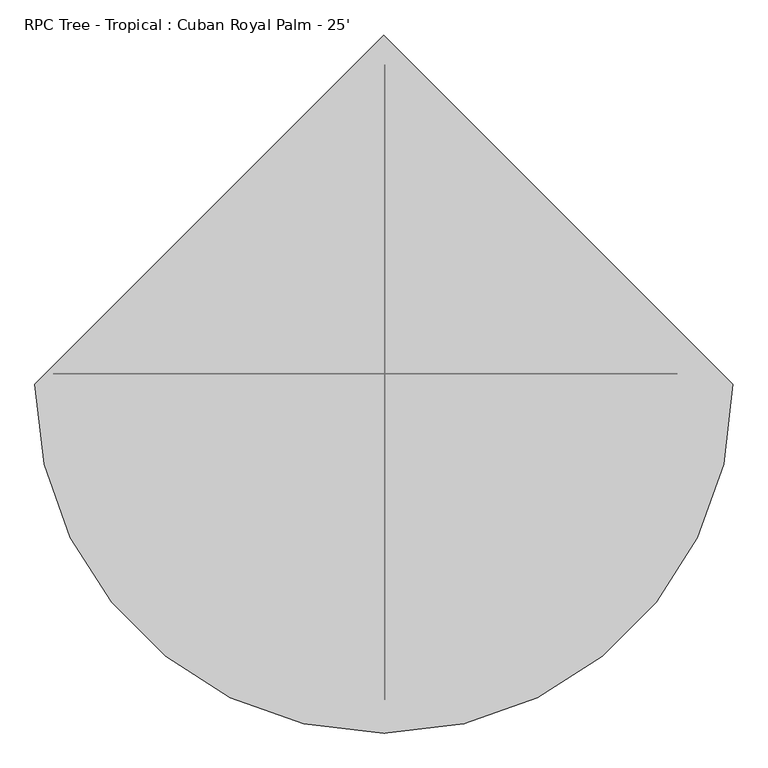
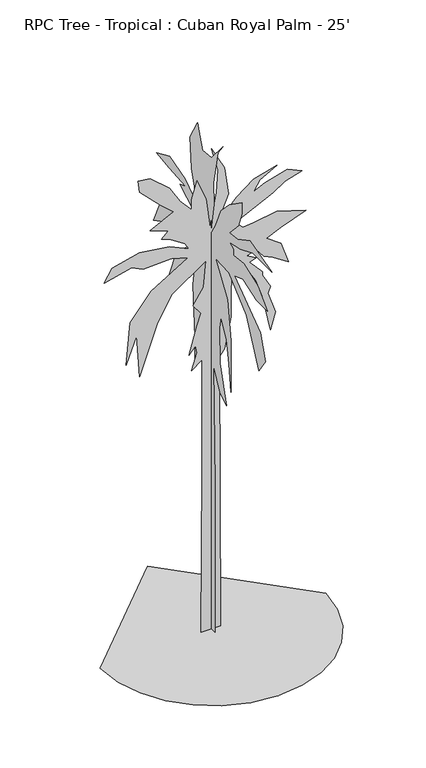
"""IFC4 building model written with IfcOpenShell, lengths in millimetres: geographic element geometry, RPC Tree - Tropical : Cuban Royal Palm - 25'."""

from ifc_helpers import new_model, si_unit, origin, place, context, project, spatial, triangles, source, transform, mapped, element, save


def rpc_tree_tropical_cuban_royal_palm_25_6f0ceb55(model_context):
    return source(origin(), model_context, "Body", "Tessellation", [
        triangles([(-54.3826135, -0.017491, 0.0009437), (-150.0419681, -0.0174994, 0.0009479), (-130.9099418, -0.0179382, 2494.6483109), (-130.9096875, -0.0182426, 4197.3711227), (-283.9640988, -0.0182154, 4082.5885941), (-207.4377743, -0.0182632, 4331.3053894), (-226.5690375, -0.0182829, 4446.0876274), (-322.2291687, -0.0182582, 4331.3053894), (-207.4375199, -0.0183385, 4752.2081863), (-150.0417137, -0.0183718, 4924.3947693), (-264.8328356, -0.0183942, 5077.4551941), (-111.778179, -0.0184419, 5307.0196701), (-73.5143854, -0.0185154, 5708.7968903), (-570.9431663, -0.0184321, 5364.4237244), (-781.3921303, -0.0183579, 5000.9249817), (-1049.2399527, -0.0182128, 4254.775177), (-1087.5024427, -0.0183274, 4905.2686111), (-1240.5575626, -0.0182489, 4503.4916817), (-1183.1638275, -0.0183643, 5134.8336685), (-877.0535151, -0.0184461, 5517.4841492), (-341.3604137, -0.0185277, 5842.7305756), (-590.0744476, -0.0185305, 5919.260788), (-991.8436014, -0.0185095, 5900.10905), (-1164.030039, -0.0185156, 5976.6392624), (-1565.7991928, -0.018481, 5880.9828918), (-1451.0091064, -0.0185202, 6072.2956329), (-1049.2399527, -0.0185549, 6167.9775833), (-609.2056927, -0.0185639, 6110.5735291), (-322.2291687, -0.0185524, 5976.6392624), (-379.6254836, -0.018567, 6072.2956329), (-609.2056927, -0.0185844, 6225.3560577), (-723.9983225, -0.0185862, 6263.6339539), (-628.3394812, -0.0186075, 6359.2903244), (-896.1847601, -0.0186129, 6454.9461136), (-551.8119212, -0.0186587, 6627.1326965), (-743.1295675, -0.0186811, 6799.3192795), (-1049.2399527, -0.0187225, 7105.4395477), (-1068.3711977, -0.0187524, 7277.6261307), (-896.1847601, -0.0187566, 7258.4743927), (-609.2056927, -0.0187246, 7009.7581787), (-456.1505364, -0.0186868, 6761.0413834), (-283.9640988, -0.0186602, 6569.7286423), (-283.9640988, -0.0186875, 6722.7890671), (-207.4375199, -0.0187388, 6990.6320206), (-73.5143854, -0.0186865, 6665.3850128), (-16.1188494, -0.0186069, 6206.2298996), (79.5405301, -0.0187, 6703.6629089), (98.6725473, -0.0187624, 7048.0354935), (3.0131737, -0.0188232, 7411.5348175), (194.3319064, -0.0187666, 7048.0354935), (251.7277126, -0.0186938, 6627.1326965), (79.5405301, -0.018611, 6206.2298996), (366.5190888, -0.0186818, 6531.476326), (615.2330864, -0.0187268, 6722.7890671), (959.6059616, -0.018759, 6818.4454376), (710.8919277, -0.0187242, 6684.5367508), (615.2330864, -0.0186926, 6531.476326), (787.419524, -0.0187138, 6608.0065384), (1112.6611542, -0.0187452, 6703.6629089), (1323.1125526, -0.0187373, 6608.0065384), (1074.3985914, -0.0187127, 6531.476326), (902.2121538, -0.0186847, 6416.6687988), (347.3878438, -0.0186125, 6148.8258453), (462.1779302, -0.018597, 6034.0433167), (615.2330864, -0.0186071, 6053.1694748), (959.6059616, -0.0186324, 6110.5735291), (1380.5089039, -0.0186269, 5976.6392624), (1017.0023129, -0.018587, 5842.7305756), (806.550769, -0.0185607, 5747.074205), (1017.0023129, -0.0185426, 5594.0143616), (1131.7923992, -0.0184894, 5268.7673538), (902.2121538, -0.0185068, 5421.8277786), (768.288279, -0.0185112, 5479.2062531), (615.2330864, -0.0185387, 5670.544574), (615.2330864, -0.0185284, 5613.1405197), (519.5742451, -0.0185174, 5574.8882034), (653.4956491, -0.0185096, 5498.357991), (557.8367715, -0.0184985, 5460.0800949), (749.1570339, -0.0184693, 5249.6411957), (749.1570339, -0.018459, 5192.2371414), (863.9471203, -0.0184264, 4981.7988235), (825.6846302, -0.0184076, 4886.142453), (940.4747166, -0.0183545, 4560.8957359), (863.9471203, -0.0183067, 4312.1792313), (749.1570339, -0.0184009, 4866.990715), (653.4956491, -0.018448, 5153.9848251), (481.3092115, -0.0184918, 5440.9539368), (309.1227739, -0.0184979, 5517.4841492), (289.9915107, -0.0184287, 5134.8336685), (289.9915107, -0.0183534, 4713.9558701), (194.3319064, -0.0182671, 4254.775177), (117.8043192, -0.0182467, 4159.1188065), (136.9360911, -0.0175052, 0.0009354), (-0.003708, 89.5986644, 0.000495), (-0.0037084, 163.6334895, 0.0005082), (-0.003708, 163.6334895, 1826.7789024), (-0.003706, 145.1250443, 4288.4300995), (-0.0037076, 219.1593699, 4177.3813545), (-0.0037057, 404.2456741, 3788.6856033), (-0.0037071, 404.2456741, 4251.4224747), (-0.0037068, 459.7725537, 5028.7883972), (-0.0037083, 385.7367022, 5565.5410995), (-0.0037091, 533.8058619, 5398.9425476), (-0.0037068, 792.9287807, 4862.190136), (-0.0037064, 1089.0671001, 4492.0362762), (-0.0037084, 1311.1695316, 4140.3737297), (-0.0037071, 1052.0491562, 4843.6988228), (-0.0037074, 885.4710245, 5250.8858871), (-0.0037074, 515.2968899, 5621.065036), (-0.003709, 681.8750216, 5584.0318314), (-0.0037073, 903.9799965, 5565.5410995), (-0.0037076, 1107.5760721, 5602.5487244), (-0.0037076, 1459.2413074, 5417.4588593), (-0.0037087, 1274.1542038, 5824.6462143), (-0.0037067, 1070.5581282, 5824.6462143), (-0.0037071, 996.5223129, 6139.3008453), (-0.0037076, 644.859621, 6065.2600159), (-0.0037089, 422.7546461, 6176.3084702), (-0.0037091, 792.9287807, 6379.9146469), (-0.0037059, 644.859621, 6435.4391647), (-0.0037081, 1052.0491562, 6472.4467896), (-0.0037064, 1385.2054195, 6509.4799942), (-0.0037073, 1052.0491562, 6657.5366547), (-0.0037075, 663.368593, 6546.487619), (-0.0037092, 348.7187945, 6324.3907104), (-0.003707, 496.7904977, 6805.6183136), (-0.0037068, 533.8058619, 7268.3296051), (-0.0037076, 348.7187945, 7601.4755493), (-0.0037068, 311.703394, 7490.427095), (-0.0037069, 219.1593699, 7249.8132935), (-0.0037086, -2.9445681, 7268.3296051), (-0.0037062, -299.0821622, 7619.9924423), (-0.0037078, -169.5227376, 7453.4194702), (-0.0037084, -58.4704863, 6916.6673492), (-0.0037085, -76.9791948, 6602.0121368), (-0.003709, 15.5640629, 6083.7763275), (-0.0037058, -113.9968663, 6287.3575058), (-0.0037085, -243.5573174, 6602.0121368), (-0.0037085, -465.6602757, 6824.1096268), (-0.003709, -780.3075308, 7046.2321152), (-0.003709, -780.3075308, 6879.6341446), (-0.0037083, -687.765287, 6639.0453415), (-0.0037091, -465.6602757, 6398.4315399), (-0.0037063, -669.256315, 6416.9228531), (-0.0037092, -983.9036064, 6583.4958252), (-0.0037074, -1539.164772, 6435.4391647), (-0.0037081, -1057.9394217, 6435.4391647), (-0.0037072, -743.2921303, 6305.8738174), (-0.0037083, -465.6602757, 6250.3492996), (-0.0037076, -558.2050993, 6194.8253632), (-0.003708, -558.2050993, 6102.2932205), (-0.0037077, -835.8344467, 6139.3008453), (-0.0037071, -1187.4996094, 6009.735498), (-0.0037064, -1428.1110855, 5769.1216965), (-0.0037087, -1150.4816654, 5769.1216965), (-0.0037066, -798.8165028, 5880.1701508), (-0.0037081, -595.2230069, 5806.1549011), (-0.0037069, -1243.0264526, 5324.9267166), (-0.0037071, -1372.586713, 4954.7475677), (-0.0037067, -1206.0085814, 4714.1337662), (-0.0037072, -891.36129, 5380.4512344), (-0.0037069, -447.1538472, 5769.1216965), (-0.003706, -113.9968663, 5787.6380081), (-0.0037066, -410.1359396, 5324.9267166), (-0.0037068, -502.6781834, 4751.141391), (-0.0037091, -502.6781834, 3955.2841553), (-0.0037069, -447.1538472, 4362.470929), (-0.003708, -391.6269676, 4695.6171638), (-0.0037083, -243.5573174, 4954.7475677), (-0.0037075, -206.5399003, 4769.6579933), (-0.0037065, -225.0485998, 4232.9058723), (-0.0037092, -391.6269676, 3677.6368584), (-0.0037079, -225.0485998, 3788.6856033), (-0.0037085, -58.4704863, 4103.3405251), (-0.0037063, -95.4881577, 2289.4952808), (-0.0037089, -95.4881577, 0.0004619), (-1653.0963352, -49.1291369, 0.0005424), (-1609.512513, -426.8745255, 0.000473), (-1485.3879673, -773.7746447, 0.0004055), (-1290.6616264, -1079.890044, 0.0003423), (-1035.2724913, -1335.2792519, 0.0002854), (-729.1570919, -1530.0055927, 0.0002372), (-382.2594435, -1654.1301384, 0.0001999), (-4.5121786, -1697.7139606, 0.0001756), (373.234849, -1654.1301384, 0.0001668), (720.1324247, -1530.0055927, 0.0001739), (1026.2478968, -1335.2792519, 0.0001953), (1281.6370319, -1079.890044, 0.0002298), (1476.3633728, -773.7746447, 0.000276), (1600.4879185, -426.8745255, 0.0003326), (1644.0717407, -49.1291369, 0.0003983), (-4.5124832, 1599.4541153, 0.0003027)], [[54, 55, 56], [48, 49, 50], [17, 18, 19], [15, 16, 17], [7, 8, 9], [83, 84, 85], [82, 83, 85], [4, 5, 6], [70, 71, 72], [66, 67, 68], [43, 44, 45], [59, 60, 61], [24, 25, 26], [24, 26, 27], [33, 34, 35], [76, 77, 78], [58, 59, 61], [58, 61, 62], [31, 32, 33], [42, 43, 45], [42, 45, 46], [37, 38, 39], [54, 56, 57], [53, 54, 57], [23, 24, 27], [23, 27, 28], [22, 23, 28], [22, 28, 29], [21, 22, 29], [58, 62, 63], [57, 58, 63], [53, 57, 63], [52, 53, 63], [36, 37, 39], [36, 39, 40], [36, 40, 41], [35, 36, 41], [35, 41, 42], [69, 70, 72], [69, 72, 73], [69, 73, 74], [65, 66, 68], [65, 68, 69], [65, 69, 74], [64, 65, 74], [47, 48, 50], [47, 50, 51], [46, 47, 51], [46, 51, 52], [33, 35, 42], [82, 85, 86], [81, 82, 86], [80, 81, 86], [33, 42, 46], [31, 33, 46], [30, 31, 46], [29, 30, 46], [15, 17, 19], [15, 19, 20], [14, 15, 20], [14, 20, 21], [13, 14, 21], [92, 93, 1], [92, 1, 2], [92, 2, 3], [92, 3, 4], [80, 86, 87], [79, 80, 87], [78, 79, 87], [76, 78, 87], [76, 87, 88], [13, 21, 29], [13, 29, 46], [13, 46, 52], [13, 52, 63], [13, 63, 64], [13, 64, 74], [13, 74, 75], [13, 75, 76], [13, 76, 88], [12, 13, 88], [12, 88, 89], [11, 12, 89], [10, 11, 89], [10, 89, 90], [9, 10, 90], [9, 90, 91], [7, 9, 91], [6, 7, 91], [4, 6, 91], [92, 4, 91], [131, 132, 133], [165, 166, 167], [105, 106, 107], [145, 146, 147], [165, 167, 168], [98, 99, 100], [131, 133, 134], [121, 122, 123], [104, 105, 107], [112, 113, 114], [171, 172, 173], [171, 173, 174], [153, 154, 155], [127, 128, 129], [118, 119, 120], [112, 114, 115], [139, 140, 141], [139, 141, 142], [159, 160, 161], [158, 159, 161], [157, 158, 161], [157, 161, 162], [104, 107, 108], [103, 104, 108], [103, 108, 109], [102, 103, 109], [127, 129, 130], [121, 123, 124], [120, 121, 124], [120, 124, 125], [118, 120, 125], [153, 155, 156], [152, 153, 156], [151, 152, 156], [151, 156, 157], [126, 127, 130], [145, 147, 148], [144, 145, 148], [144, 148, 149], [143, 144, 149], [139, 142, 143], [138, 139, 143], [137, 138, 143], [137, 143, 149], [175, 176, 94], [175, 94, 95], [175, 95, 96], [175, 96, 97], [174, 175, 97], [111, 112, 115], [115, 116, 117], [111, 115, 117], [110, 111, 117], [109, 110, 117], [165, 168, 169], [164, 165, 169], [130, 131, 134], [126, 130, 134], [126, 134, 135], [125, 126, 135], [125, 135, 136], [118, 125, 136], [151, 157, 162], [171, 174, 97], [170, 171, 97], [109, 117, 118], [109, 118, 136], [102, 109, 136], [97, 98, 100], [97, 100, 101], [170, 97, 101], [169, 170, 101], [169, 101, 102], [164, 169, 102], [163, 164, 102], [163, 102, 136], [151, 162, 163], [151, 163, 136], [151, 136, 137], [151, 137, 149], [151, 149, 150], [191, 192, 177], [190, 191, 177], [190, 177, 178], [189, 190, 178], [189, 178, 179], [189, 179, 180], [188, 189, 180], [187, 188, 180], [187, 180, 181], [187, 181, 182], [187, 182, 183], [187, 183, 184], [187, 184, 185], [187, 185, 186]], closed=False),
    ])


if __name__ == "__main__":
    model = new_model("IFC4")
    model_context = context("Model", 3, world=origin())
    ifc_project = project(units=[si_unit("LENGTHUNIT", "METRE", prefix="MILLI")], contexts=[model_context])
    site = spatial("IfcSite", under=ifc_project)
    building = spatial("IfcBuilding", under=site)
    placement = place(None, origin())
    rpc_tree_tropical_cuban_royal_palm_25_shape = rpc_tree_tropical_cuban_royal_palm_25_6f0ceb55(model_context)
    element("IfcGeographicElement", 1, ObjectType="RPC Tree - Tropical : Cuban Royal Palm - 25'", at=placement, inside=building, context=model_context, shape_type="MappedRepresentation", body=[
        mapped(rpc_tree_tropical_cuban_royal_palm_25_shape, transform((0.0, 0.0, 0.0), x_axis=(1.0, 0.0, 0.0), y_axis=(0.0, 1.0, 0.0), z_axis=(0.0, 0.0, 1.0))),
    ])
    save(model, "model.ifc")

# Revit data of these elements
# Type "RPC Tree - Tropical : Cuban Royal Palm - 25'"
#   built-in parameter 1005198 = "{2, 15},{39, RPC-16-FVGV-NKG0-7NHH-C000-ST1L-LVER-AU},{1, 0},{1, 0},{2, 35},{1, 8},{5, Color},{1, 0},{1, 0},{3, 0.8},{3, 0.8},{3, 0.8},{1, 8},{7, BBoxMin},{1, 0},{1, 0},{1, 0},{1, 0},{1, 0},{1, 8},{7, BBoxMax},{1, 0},{1, 0},{1, 0},{1, 0},{1, 0},{2, 11},{9, RPCTypeId},{1, 0},{1, 0},{39, RPC-16-FVGV-NKG0-7NHH-C000-ST1L-LVER-AU},{1, 6},{14, RPCPlantHeight},{1, 0},{1, 0},{2, 25},{2, 11},{7, keyword},{1, 0},{1, 0},{72, :Geometry:RPC:Cuban Royal Palm:Roystonea regia (Oreodoxa):palm:tropical.},{2, 11},{8, category},{1, 0},{1, 0},{17, :Trees [Tropical]},{2, 11},{12, LocalizedUID},{1, 0},{1, 0},{16, Cuban Royal Palm},{2, 14},{6, Height},{1, 0},{1, 0},{2, 25},{1, 2},{16, Cast Reflections},{1, 0},{1, 0},{1, 0},{1, 2},{12, Cast Shadows},{1, 0},{1, 0},{1, 1},{1, 2},{9, Lock View},{1, 0},{1, 0},{1, 0},{1, 4},{5, ViewC},{1, 0},{1, 0},{1, 0},{2, 11},{20, AdvancedUIDefinition},{1, 0},{1, 0},{0, },{2, 11},{10, AssetLibID},{1, 0},{1, 0},{36, 4D3F6E72-3F99-4203-98E9-AF80B3C7A7A4},{2, 11},{10, BaseSchema},{1, 0},{1, 0},{9, RPCSchema},{2, 11},{12, ExchangeGUID},{1, 0},{1, 0},{0, },{1, 2},{6, Hidden},{1, 0},{1, 0},{1, 0},{1, 4},{11, RPCCategory},{1, 0},{1, 0},{1, 0},{2, 11},{8, RPCImage},{1, 0},{1, 0},{0, },{1, 4},{13, SchemaVersion},{1, 0},{1, 0},{1, 4},{2, 11},{12, UIDefinition},{1, 0},{1, 0},{0, },{2, 11},{6, UIName},{1, 0},{1, 0},{39, RPC-16-FVGV-NKG0-7NHH-C000-ST1L-LVER-AU},{2, 11},{11, VersionGUID},{1, 0},{1, 0},{9, RPCSchema},{2, 11},{9, assettype},{1, 0},{1, 0},{11, RPCGeometry},{2, 11},{11, description},{1, 0},{1, 0},{0, },{2, 11},{9, localname},{1, 0},{1, 0},{3, RPC},{2, 11},{9, localtype},{1, 0},{1, 0},{3, RPC},{1, 4},{8, revision},{1, 0},{1, 0},{1, 1},{2, 11},{9, thumbnail},{1, 0},{1, 0},{0, },{1, 4},{7, version},{1, 0},{1, 0},{1, 1},{1, 2},{20, RPC_Cast Reflections},{1, 0},{1, 0},{1, 1},{1, 2},{16, RPC_Cast Shadows},{1, 0},{1, 0},{1, 1},{1, 2},{13, RPC_Lock View},{1, 0},{1, 0},{1, 0},{1, 4},{9, RPC_ViewC},{1, 0},{1, 0},{1, 0},{21, assetlibrary_base.fbx},{1, 5},"
#   built-in parameter 1005195 = "RPC-16-FVGV-NKG0-7NHH-C000-ST1L-LVER-AU"
#   Type Comments = "Cuban Royal Palm"
#   Assembly Code = "G2050500"
#   Height = 25' - 0"
#   Plan Symbol = element 455244
#   Default Elevation = 0
